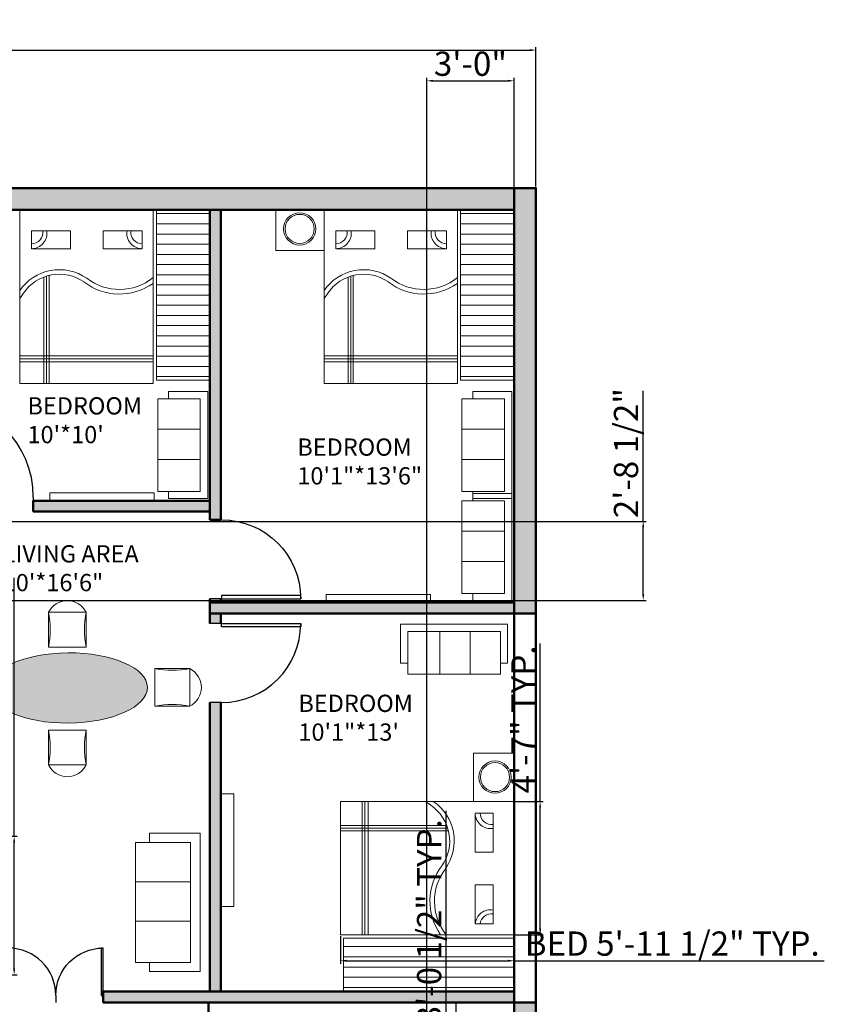
# Model space of a CAD drawing. Units: inches. Extents: x 1477 to 2233, y 1388 to 2326.
# Tile 4 of 4: x 1901 to 2233, y 1870 to 2277. Entities that reach past the tile are written whole.
import ezdxf

# ---------------------------------------------------------------- set-up
doc = ezdxf.new("R2010")
doc.units = ezdxf.units.IN
for name, color, linetype, lineweight in [('A-ANNO-DIMS', 2, 'Continuous', 18), ('A-AREA-IDEN', 7, 'Continuous', 18), ('A-DOOR', 4, 'Continuous', 25), ('A-EQPM', 8, 'Continuous', 18), ('A-FLOR-CASE', 9, 'Continuous', 25), ('A-FURN-PATT', 9, 'Continuous', 13), ('A-WALL-PATT', 10, 'Continuous', 13), ('bed', 200, 'Continuous', 18), ('book', 104, 'Continuous', 18), ('dining', 220, 'Continuous', 18), ('sofa', 130, 'Continuous', 18), ('table', 40, 'Continuous', 18), ('wall', 10, 'Continuous', 50)]:
    doc.layers.add(name, color=color, linetype=linetype, lineweight=lineweight)
doc.styles.get("Standard").update_dxf_attribs({"font": 'arial.ttf'})
doc.dimstyles.new('ISO-25', dxfattribs={"dimtxt": 10, "dimasz": 2.5, "dimexe": 1.25, "dimexo": 0.625, "dimtad": 1, "dimdec": 0, "dimlunit": 4, "dimtxsty": 'Standard', "dimcen": 2.5, "dimadec": 0, "dimazin": 0, "dimtfac": 1, "dimtdec": 0, "dimtmove": 0, "dimatfit": 3, "dimfxl": 1, "dimarcsym": 0})

# ---------------------------------------------------------------- blocks, each defined once
blk = doc.blocks.new('*U2')
for p, q in [((0, 0), (0, -6)), ((40, 0), (40, -6))]:
    blk.add_line(p, q)
blk.add_lwpolyline([(0, 0), (0, 40), (1.75, 40), (1.75, 0)], close=True)
blk.add_arc((0, 0), 40, 0, 90)
blk = doc.blocks.new('*D4')
at = {"layer": 'A-ANNO-DIMS', "color": 0, "lineweight": -2, "transparency": 16777216}
for p, q in [((1601.11, 2207.8), (1601.11, 2265.33)), ((1603.61, 2264.08), (2111.11, 2264.08)), ((2113.61, 2207.8), (2113.61, 2265.33))]:
    blk.add_line(p, q, dxfattribs=at)
at = {"layer": 'A-ANNO-DIMS', "color": 0, "transparency": 16777216}
for points in [[(1603.61, 2264.5), (1603.61, 2263.66), (1601.11, 2264.08)], [(2111.11, 2264.5), (2111.11, 2263.66), (2113.61, 2264.08)]]:
    blk.add_solid(points, dxfattribs=at)
at = {"layer": 'Defpoints', "color": 0, "transparency": 16777216}
for p in [(2113.61, 2264.08), (1601.11, 2207.17), (2113.61, 2207.17)]:
    blk.add_point(p, dxfattribs=at)
at = {"layer": 'A-ANNO-DIMS', "color": 0, "transparency": 16777216, "insert": (1857.36, 2269.81), "char_height": 10, "attachment_point": 5}
blk.add_mtext('42\'-9"', dxfattribs=at)
blk = doc.blocks.new('BED-DOUBLE')
for p, q in [((42.9, 44.24), (42.9, 44.54)), ((42.9, 44.24), (42.9, 0)), ((43.98, 44.24), (43.98, 0)), ((45.09, 43.85), (45.09, 0)), ((53.44, 37.23), (54.99, 35.03)), ((0, 11.42), (54.99, 11.42)), ((0, 10.1), (54.99, 10.1)), ((0, 8.97), (54.99, 8.97))]:
    blk.add_line(p, q)
for points in [[(0, 71.61), (54.99, 71.61), (54.99, 0), (0, 0)], [(4.46, 63.01), (20.6, 63.01), (20.6, 55.57), (4.46, 55.57)], [(50.13, 63.01), (34, 63.01), (34, 55.57), (50.13, 55.57)]]:
    blk.add_lwpolyline(points, close=True)
for centre, radius, start, end in [((4.46, 61.93), 6.36, 270, 9.8305), ((4.46, 62.26), 4.68, 270, 9.2541), ((50.13, 61.93), 6.36, 170.1695, 270), ((50.13, 62.26), 4.68, 170.7459, 270), ((38.65, 27.17), 19.76, 34.2245, 124.798), ((38.65, 27.17), 17.88, 34.2245, 124.798), ((13.85, 60.88), 22.1, 231.1871, 307.7214), ((13.85, 60.88), 23.99, 234.7235, 307.7214)]:
    blk.add_arc(centre, radius, start, end)
blk = doc.blocks.new('BED-DOUBLE-ALT')
for p, q in [((8.97, 0), (8.97, 54.99)), ((10.1, 0), (10.1, 54.99)), ((11.42, 0), (11.42, 54.99)), ((37.23, 53.44), (35.03, 54.99)), ((43.85, 45.09), (0, 45.09)), ((44.24, 43.98), (0, 43.98)), ((44.24, 42.9), (0, 42.9)), ((44.24, 42.9), (44.54, 42.9))]:
    blk.add_line(p, q)
for points in [[(71.61, 0), (71.61, 54.99), (0, 54.99), (0, 0)], [(63.01, 50.13), (63.01, 34), (55.57, 34), (55.57, 50.13)], [(63.01, 4.46), (63.01, 20.6), (55.57, 20.6), (55.57, 4.46)]]:
    blk.add_lwpolyline(points, close=True)
for centre, radius, start, end in [((27.17, 38.65), 17.88, 325.202, 55.7755), ((27.17, 38.65), 19.76, 325.202, 55.7755), ((61.93, 50.13), 6.36, 180, 279.8305), ((62.26, 50.13), 4.68, 180, 279.2541), ((60.88, 13.85), 23.99, 142.2786, 215.2765), ((60.88, 13.85), 22.1, 142.2786, 218.8129), ((61.93, 3.93), 6.36, 80.1695, 175.1865), ((62.26, 3.93), 4.68, 80.7459, 173.4549)]:
    blk.add_arc(centre, radius, start, end)
blk = doc.blocks.new('NIGHTSTAND-LAMP')
blk.add_lwpolyline([(0, 16.8), (19.92, 16.8), (19.92, 0), (0, 0)], close=True)
for radius in [6.66, 6]:
    blk.add_circle((10.02, 8.94), radius)
blk = doc.blocks.new('SOFA-COMPACT-ALT')
for p, q in [((0, 4.5), (0, 20.62)), ((0, 20.62), (44.13, 20.62)), ((44.13, 4.5), (44.13, 20.62)), ((16.11, 17.56), (16.11, 0)), ((28.61, 17.56), (28.61, 0)), ((2.91, 4.5), (0, 4.5)), ((1.29, 4.5), (2.91, 4.5)), ((41.13, 4.5), (44.13, 4.5))]:
    blk.add_line(p, q)
blk.add_lwpolyline([(2.91, 0), (2.91, 17.56), (41.13, 17.56), (41.13, 0)], close=True)
blk = doc.blocks.new('SOFA-STANDARD-ALT')
for p, q in [((0, 26.7), (57.14, 26.7)), ((0, 26.7), (0, 5.83)), ((57.14, 5.83), (57.14, 26.7)), ((20.86, 22.74), (20.86, 0)), ((37.04, 22.74), (37.04, 0)), ((3.76, 5.83), (0, 5.83)), ((53.26, 5.83), (57.14, 5.83))]:
    blk.add_line(p, q)
blk.add_lwpolyline([(3.76, 0), (3.76, 22.74), (53.26, 22.74), (53.26, 0)], close=True)
blk = doc.blocks.new('CHAIR-DINING')
blk.add_lwpolyline([(0, 0), (15.48, 0), (15.48, 14.4), (0, 14.4)], close=True)
for centre, radius, start, end in [((7.74, 10.64), 8.6, 25.8733, 154.1267), ((-38.59, 7.2), 39.26, 349.434, 10.566), ((53.9, 7.2), 39.09, 169.3873, 190.6127)]:
    blk.add_arc(centre, radius, start, end)
blk = doc.blocks.new('*D19')
at = {"layer": 'A-ANNO-DIMS', "color": 0, "lineweight": -2, "transparency": 16777216}
for p, q in [((1898.42, 1939.74), (1898.42, 2046.31)), ((1890.47, 1939.74), (1899.67, 1939.74)), ((1898.42, 1885.1), (1898.42, 1937.24)), ((1890.47, 1882.6), (1899.67, 1882.6))]:
    blk.add_line(p, q, dxfattribs=at)
at = {"layer": 'A-ANNO-DIMS', "color": 0, "transparency": 16777216}
for points in [[(1898, 1937.24), (1898.83, 1937.24), (1898.42, 1939.74)], [(1898, 1885.1), (1898.83, 1885.1), (1898.42, 1882.6)]]:
    blk.add_solid(points, dxfattribs=at)
at = {"layer": 'Defpoints', "color": 0, "transparency": 16777216}
for p in [(1889.85, 1939.74), (1898.42, 1939.74), (1889.85, 1882.6)]:
    blk.add_point(p, dxfattribs=at)
at = {"layer": 'A-ANNO-DIMS', "color": 0, "transparency": 16777216, "insert": (1892.62, 1994.27), "char_height": 10, "attachment_point": 5, "rotation": 90}
blk.add_mtext('SOFA 4\'-9" TYP.', dxfattribs=at)
blk = doc.blocks.new('*D25')
at = {"layer": 'A-ANNO-DIMS', "color": 0, "lineweight": -2, "transparency": 16777216}
for p, q in [((2033, 1898.51), (2033, 1887.14)), ((2104.61, 1898.51), (2104.61, 1887.14)), ((2035.5, 1888.39), (2102.11, 1888.39)), ((2104.61, 1888.39), (2232.55, 1888.39))]:
    blk.add_line(p, q, dxfattribs=at)
at = {"layer": 'A-ANNO-DIMS', "color": 0, "transparency": 16777216}
for points in [[(2035.5, 1888.81), (2035.5, 1887.97), (2033, 1888.39)], [(2102.11, 1888.81), (2102.11, 1887.97), (2104.61, 1888.39)]]:
    blk.add_solid(points, dxfattribs=at)
at = {"layer": 'Defpoints', "color": 0, "transparency": 16777216}
for p in [(2033, 1899.13), (2104.61, 1899.13), (2104.61, 1888.39)]:
    blk.add_point(p, dxfattribs=at)
at = {"layer": 'A-ANNO-DIMS', "color": 0, "transparency": 16777216, "insert": (2169.83, 1894.18), "char_height": 10, "attachment_point": 5}
blk.add_mtext('BED 5\'-11 1/2" TYP.', dxfattribs=at)
blk = doc.blocks.new('*D26')
at = {"layer": 'A-ANNO-DIMS', "color": 0, "lineweight": -2, "transparency": 16777216}
for p, q in [((2115.35, 1954.13), (2115.35, 2019.23)), ((2105.23, 1954.13), (2116.6, 1954.13)), ((2115.35, 1901.63), (2115.35, 1951.63)), ((2105.23, 1899.13), (2116.6, 1899.13))]:
    blk.add_line(p, q, dxfattribs=at)
at = {"layer": 'A-ANNO-DIMS', "color": 0, "transparency": 16777216}
for points in [[(2114.93, 1951.63), (2115.77, 1951.63), (2115.35, 1954.13)], [(2114.93, 1901.63), (2115.77, 1901.63), (2115.35, 1899.13)]]:
    blk.add_solid(points, dxfattribs=at)
at = {"layer": 'Defpoints', "color": 0, "transparency": 16777216}
for p in [(2104.61, 1954.13), (2115.35, 1954.13), (2104.61, 1899.13)]:
    blk.add_point(p, dxfattribs=at)
at = {"layer": 'A-ANNO-DIMS', "color": 0, "transparency": 16777216, "insert": (2109.72, 1987.93), "char_height": 10, "attachment_point": 5, "rotation": 90}
blk.add_mtext('4\'-7" TYP.', dxfattribs=at)
blk = doc.blocks.new('*D29')
at = {"layer": 'A-ANNO-DIMS', "color": 0, "lineweight": -2, "transparency": 16777216}
for p, q in [((2076.64, 1799.12), (2076.64, 1950.21)), ((2081.48, 1799.12), (2075.39, 1799.12)), ((2076.64, 1765.24), (2076.64, 1796.62)), ((2081.48, 1762.74), (2075.39, 1762.74))]:
    blk.add_line(p, q, dxfattribs=at)
at = {"layer": 'A-ANNO-DIMS', "color": 0, "transparency": 16777216}
for points in [[(2076.23, 1796.62), (2077.06, 1796.62), (2076.64, 1799.12)], [(2076.23, 1765.24), (2077.06, 1765.24), (2076.64, 1762.74)]]:
    blk.add_solid(points, dxfattribs=at)
at = {"layer": 'Defpoints', "color": 0, "transparency": 16777216}
for p in [(2076.64, 1799.12), (2082.1, 1799.12), (2082.1, 1762.74)]:
    blk.add_point(p, dxfattribs=at)
at = {"layer": 'A-ANNO-DIMS', "color": 0, "transparency": 16777216, "insert": (2070.85, 1875.92), "char_height": 10, "attachment_point": 5, "rotation": 90}
blk.add_mtext('FIXTURE 3\'-0 1/2" TYP.', dxfattribs=at)
blk = doc.blocks.new('*D35')
at = {"layer": 'A-ANNO-DIMS', "color": 0, "lineweight": -2, "transparency": 16777216}
for p, q in [((2068.61, 1625.95), (2068.61, 2252.67)), ((2071.11, 2251.42), (2102.11, 2251.42)), ((2104.61, 1625.66), (2104.61, 2252.67))]:
    blk.add_line(p, q, dxfattribs=at)
at = {"layer": 'A-ANNO-DIMS', "color": 0, "transparency": 16777216}
for points in [[(2071.11, 2251.84), (2071.11, 2251.01), (2068.61, 2251.42)], [(2102.11, 2251.84), (2102.11, 2251.01), (2104.61, 2251.42)]]:
    blk.add_solid(points, dxfattribs=at)
at = {"layer": 'Defpoints', "color": 0, "transparency": 16777216}
for p in [(2104.61, 2251.42), (2068.61, 1625.33), (2104.61, 1625.03)]:
    blk.add_point(p, dxfattribs=at)
at = {"layer": 'A-ANNO-DIMS', "color": 0, "transparency": 16777216, "insert": (2086.61, 2257.16), "char_height": 10, "attachment_point": 5}
blk.add_mtext('3\'-0"', dxfattribs=at)
blk = doc.blocks.new('*D37')
at = {"layer": 'A-ANNO-DIMS', "color": 0, "lineweight": -2, "transparency": 16777216}
for p, q in [((2080.61, 1870.55), (2080.61, 1395.67)), ((2104.61, 1870.55), (2104.61, 1395.67)), ((2083.11, 1396.92), (2102.11, 1396.92)), ((2104.61, 1396.92), (2135.11, 1396.92))]:
    blk.add_line(p, q, dxfattribs=at)
at = {"layer": 'A-ANNO-DIMS', "color": 0, "transparency": 16777216}
for points in [[(2083.11, 1397.34), (2083.11, 1396.51), (2080.61, 1396.92)], [(2102.11, 1397.34), (2102.11, 1396.51), (2104.61, 1396.92)]]:
    blk.add_solid(points, dxfattribs=at)
at = {"layer": 'Defpoints', "color": 0, "transparency": 16777216}
for p in [(2080.61, 1871.17), (2104.61, 1871.17), (2104.61, 1396.92)]:
    blk.add_point(p, dxfattribs=at)
at = {"layer": 'A-ANNO-DIMS', "color": 0, "transparency": 16777216, "insert": (2121.11, 1402.65), "char_height": 10, "attachment_point": 5}
blk.add_mtext('2\'-0"', dxfattribs=at)
blk = doc.blocks.new('*D40')
at = {"layer": 'A-ANNO-DIMS', "color": 0, "lineweight": -2, "transparency": 16777216}
for p, q in [((2157.86, 2069.66), (2157.86, 2123.47)), ((1730.73, 2069.66), (2159.11, 2069.66)), ((2157.86, 2039.56), (2157.86, 2067.16)), ((1730.73, 2037.06), (2159.11, 2037.06))]:
    blk.add_line(p, q, dxfattribs=at)
at = {"layer": 'A-ANNO-DIMS', "color": 0, "transparency": 16777216}
for points in [[(2157.44, 2067.16), (2158.27, 2067.16), (2157.86, 2069.66)], [(2157.44, 2039.56), (2158.27, 2039.56), (2157.86, 2037.06)]]:
    blk.add_solid(points, dxfattribs=at)
at = {"layer": 'Defpoints', "color": 0, "transparency": 16777216}
for p in [(1730.11, 2069.66), (2157.86, 2069.66), (1730.11, 2037.06)]:
    blk.add_point(p, dxfattribs=at)
at = {"layer": 'A-ANNO-DIMS', "color": 0, "transparency": 16777216, "insert": (2152.06, 2097.82), "char_height": 10, "attachment_point": 5, "rotation": 90}
blk.add_mtext('2\'-8 1/2"', dxfattribs=at)

msp = doc.modelspace()

# ---------------------------------------------------------------- hatches: boundary and pattern name
at = {"layer": 'A-FURN-PATT'}
h = msp.add_hatch(dxfattribs=at)
h.set_pattern_fill('_USER', color=256, scale=4.2, pattern_type=0)
h.set_pattern_definition([(0, (0, 0), (0, 4.2), [])])
h.paths.add_polyline_path([(1632.2, 2197.32), (1610.11, 2197.32), (1610.11, 2127.01), (1632.2, 2127.01)])
h.paths.add_polyline_path([(1757.03, 2198.17), (1734.93, 2198.17), (1734.93, 2127.87), (1757.03, 2127.87)])
h.paths.add_polyline_path([(1979.11, 2198.17), (1957.06, 2198.17), (1957.06, 2127.87), (1979.11, 2127.87)])
h.paths.add_polyline_path([(2104.61, 2198.17), (2082.56, 2198.17), (2082.56, 2127.87), (2104.61, 2127.87)])
h.paths.add_polyline_path([(2104.61, 1897.77), (2034.3, 1897.77), (2034.3, 1875.67), (2104.61, 1875.67)])
h.paths.add_polyline_path([(1680.41, 1898.15), (1610.11, 1898.15), (1610.11, 1876.06), (1680.41, 1876.06)])
h.paths.add_polyline_path([(1680.41, 1869.67), (1610.11, 1869.67), (1610.11, 1847.57), (1680.41, 1847.57)])
h.paths.add_polyline_path([(1632.2, 1521.19), (1610.11, 1521.19), (1610.11, 1450.88), (1632.2, 1450.88)])
h.paths.add_polyline_path([(1854.34, 1520.43), (1832.24, 1520.43), (1832.24, 1450.17), (1854.34, 1450.17)])
h = msp.add_hatch(color=256, dxfattribs=at)
h.dxf.hatch_style = 1
edge = h.paths.add_edge_path()
edge.add_ellipse((1794.61, 1999.29), major_axis=(32.65, 0.27), ratio=0.443592, start_angle=0, end_angle=360)
edge = h.paths.add_edge_path()
edge.add_ellipse((1920.72, 2000.93), major_axis=(32.65, 0.27), ratio=0.443592, start_angle=0, end_angle=360)
edge = h.paths.add_edge_path()
edge.add_ellipse((1854.61, 1811.96), major_axis=(32.65, 0.27), ratio=0.443592, start_angle=0, end_angle=360)
edge = h.paths.add_edge_path()
edge.add_ellipse((1749.3, 1659.55), major_axis=(32.65, 0.27), ratio=0.443592, start_angle=0, end_angle=360)
at = {"layer": 'A-WALL-PATT'}
h = msp.add_hatch(color=256, dxfattribs=at)
h.dxf.hatch_style = 1
h.paths.add_polyline_path([(2104.61, 2036.17), (1979.11, 2036.17), (1979.11, 2031.67), (2104.61, 2031.67)])
h.paths.add_polyline_path([(1983.61, 2031.67), (1979.11, 2031.67), (1979.11, 2027.53), (1983.61, 2027.53)])
h.paths.add_polyline_path([(1983.61, 2037.7), (1979.11, 2037.7), (1979.11, 2036.17), (1983.61, 2036.17)])
h.paths.add_polyline_path([(2113.61, 2207.17), (2104.61, 2207.17), (2104.61, 2031.67), (2113.61, 2031.67)])
h.paths.add_polyline_path([(2104.61, 2207.17), (1859.11, 2207.17), (1859.11, 2198.17), (2104.61, 2198.17)])
h.paths.add_polyline_path([(1983.61, 2198.17), (1979.16, 2198.17), (1979.16, 2127.87), (1979.11, 2070.31), (1983.61, 2070.31)])
h.paths.add_polyline_path([(1979.11, 2078.17), (1906.33, 2078.17), (1906.33, 2073.67), (1979.11, 2073.67)])
h.paths.add_polyline_path([(1859.11, 2198.17), (1854.61, 2198.17), (1854.61, 2078.17), (1859.11, 2078.17)])
h.paths.add_polyline_path([(1866.33, 2078.17), (1848.79, 2078.17), (1848.79, 2073.67), (1866.33, 2073.67)])
h.paths.add_polyline_path([(1859.11, 2207.17), (1734.61, 2207.17), (1734.61, 2198.17), (1859.11, 2198.17)])
h.paths.add_polyline_path([(1734.61, 2207.17), (1601.11, 2207.17), (1601.11, 2198.17), (1610.11, 2198.17), (1734.61, 2198.17)])
h.paths.add_polyline_path([(1734.61, 2198.17), (1730.11, 2198.17), (1730.11, 2069.66), (1734.61, 2069.66)])
h.paths.add_polyline_path([(1808.79, 2078.17), (1734.61, 2078.17), (1734.61, 2073.67), (1808.79, 2073.67)])
h.paths.add_polyline_path([(1610.11, 2198.17), (1601.11, 2198.17), (1601.11, 1450.43), (1610.11, 1450.43)])
h.paths.add_polyline_path([(2104.61, 1450.43), (1854.61, 1450.43), (1854.61, 1450.17), (1854.34, 1450.13), (1832.24, 1450.13), (1830.34, 1450.13), (1830.34, 1450.03), (1775.35, 1450.03), (1755.43, 1450.03), (1713.79, 1450.14), (1713.79, 1450.03), (1693.87, 1450.03), (1638.87, 1450.03), (1610.11, 1450.17), (1610.11, 1450.43), (1601.11, 1450.43), (1601.11, 1441.17), (2104.61, 1441.17)])
h.paths.add_polyline_path([(2113.61, 1871.17), (2104.61, 1871.17), (2104.61, 1441.17), (2113.61, 1441.17)])
h.paths.add_polyline_path([(1734.61, 1598.17), (1730.11, 1598.17), (1730.11, 1450.43), (1734.61, 1450.43)])
h = msp.add_hatch(color=256, dxfattribs=at)
h.dxf.hatch_style = 1
h.paths.add_polyline_path([(1734.61, 2037.06), (1730.11, 2037.06), (1730.11, 2036.17), (1610.11, 2036.17), (1610.11, 2031.67), (1734.61, 2031.67)])
h.paths.add_polyline_path([(1983.61, 1994.92), (1979.11, 1994.92), (1979.11, 1875.67), (1983.61, 1875.67)])
h = msp.add_hatch(color=256, dxfattribs=at)
h.dxf.hatch_style = 1
h.paths.add_polyline_path([(1734.61, 1993.71), (1730.11, 1993.71), (1730.11, 1875.67), (1734.61, 1875.67)])
h.paths.add_polyline_path([(1730.11, 1875.67), (1610.11, 1875.67), (1610.11, 1871.17), (1730.11, 1871.17)])
h.paths.add_polyline_path([(1776.57, 1875.67), (1730.11, 1875.67), (1730.11, 1871.17), (1776.57, 1871.17)])
h.paths.add_polyline_path([(1896.07, 1875.67), (1815.6, 1875.67), (1815.6, 1871.17), (1896.07, 1871.17)])
h.paths.add_polyline_path([(2104.61, 1875.67), (1935.11, 1875.67), (1935.11, 1871.17), (2104.61, 1871.17)])
h.paths.add_polyline_path([(1734.61, 1871.17), (1730.11, 1871.17), (1730.11, 1727.17), (1734.61, 1727.17)])
h.paths.add_polyline_path([(1775, 1727.17), (1726.93, 1727.17), (1726.93, 1722.67), (1775, 1722.67)])
h.paths.add_polyline_path([(1880.17, 1727.17), (1814.04, 1727.17), (1814.04, 1722.67), (1880.17, 1722.67)])
h.paths.add_polyline_path([(1858.61, 1722.67), (1854.11, 1722.67), (1854.12, 1598.17), (1858.61, 1598.17)])
h.paths.add_polyline_path([(1854.12, 1602.67), (1780.08, 1602.67), (1780.08, 1598.17), (1854.12, 1598.17)])
h.paths.add_polyline_path([(1740.08, 1602.67), (1722.89, 1602.67), (1722.89, 1598.17), (1740.08, 1598.17)])
h.paths.add_polyline_path([(1682.89, 1602.67), (1610.11, 1602.67), (1610.11, 1598.17), (1682.89, 1598.17)])
h.paths.add_polyline_path([(1859.11, 1598.17), (1854.61, 1598.17), (1854.61, 1450.43), (1859.11, 1450.43)])
h.paths.add_polyline_path([(2104.61, 1727.17), (1960.17, 1727.17), (1960.17, 1722.67), (2104.61, 1722.67)])
h.paths.add_polyline_path([(2104.61, 1625.03), (1978.61, 1625.03), (1978.61, 1620.53), (2104.61, 1620.53)])

# ---------------------------------------------------------------- linework, layer by layer
at = {"layer": 'A-EQPM'}
for points in [[(1956.17, 2078.17), (1913.12, 2078.17), (1913.12, 2081.42), (1956.17, 2081.42)], [(2070.17, 2036.17), (2027.12, 2036.17), (2027.12, 2039.42), (2070.17, 2039.42)], [(1983.91, 1910.78), (1989.01, 1910.78), (1989.01, 1957.26), (1983.91, 1957.26)]]:
    msp.add_lwpolyline(points, close=True, dxfattribs=at)
at = {"layer": 'A-FLOR-CASE'}
for p, q in [((2104.61, 1871.17), (2080.61, 1871.17)), ((2080.61, 1871.17), (2080.61, 1751.17))]:
    msp.add_line(p, q, dxfattribs=at)
at = {"layer": 'book'}
for points in [[(1957.06, 2198.17), (1979.16, 2198.17), (1979.16, 2127.87), (1957.06, 2127.87)], [(2082.56, 2198.17), (2104.66, 2198.17), (2104.66, 2127.87), (2082.56, 2127.87)], [(2104.61, 1897.77), (2104.61, 1875.67), (2034.3, 1875.67), (2034.3, 1897.77)]]:
    msp.add_lwpolyline(points, close=True, dxfattribs=at)
at = {"layer": 'dining'}
msp.add_ellipse((1920.72, 2000.93), major_axis=(32.65, 0.27), ratio=0.443592, dxfattribs=at)
at = {"layer": 'wall'}
for p, q in [((1859.11, 2207.17), (1983.61, 2207.17)), ((1983.61, 2207.17), (2113.61, 2207.17)), ((2113.61, 2207.17), (2113.61, 2031.67)), ((1859.11, 2198.17), (1979.11, 2198.17)), ((1979.11, 2198.17), (1979.11, 2078.17)), ((1983.61, 2198.17), (1983.61, 2073.67)), ((1983.61, 2198.17), (2104.61, 2198.17)), ((2104.61, 2198.17), (2104.61, 2036.17)), ((1979.11, 2078.17), (1979.11, 2120.13)), ((1983.61, 2070.31), (1983.61, 2120.13)), ((1979.11, 2078.17), (1906.33, 2078.17)), ((1979.11, 2073.67), (1906.33, 2073.67)), ((1979.11, 2070.31), (1979.11, 2073.67)), ((1979.11, 2031.67), (1979.11, 2037.7)), ((1983.61, 2036.17), (1983.61, 2037.7)), ((2104.61, 2036.17), (1983.61, 2036.17)), ((2113.61, 2031.67), (1979.11, 2031.67)), ((1979.11, 2027.53), (1979.11, 2031.67)), ((1983.61, 2027.53), (1983.61, 2031.67)), ((2104.61, 2031.67), (2104.61, 1875.67)), ((2113.61, 2031.67), (2113.61, 1871.17)), ((1979.11, 1875.67), (1979.11, 1994.92)), ((1983.61, 1875.67), (1983.61, 1994.92)), ((1915.53, 1875.67), (1915.65, 1875.67)), ((1934.25, 1875.67), (1993.21, 1875.67)), ((2104.61, 1875.67), (1983.61, 1875.67)), ((1935.11, 1871.17), (1981.94, 1871.17)), ((1978.61, 1727.17), (1978.61, 1871.17)), ((2113.61, 1871.17), (1979.11, 1871.17)), ((2104.61, 1871.17), (2104.61, 1727.17)), ((2113.61, 1871.17), (2113.61, 1722.67))]:
    msp.add_line(p, q, dxfattribs=at)
for points in [[(1601.11, 2207.17), (2104.61, 2207.17), (2104.61, 2198.17), (1601.11, 2198.17)], [(2104.61, 2207.17), (2113.61, 2207.17), (2113.61, 1441.17), (2104.61, 1441.17)], [(1979.11, 2070.31), (1983.61, 2070.31), (1983.61, 2198.17), (1979.11, 2198.17)], [(1906.33, 2073.67), (1979.11, 2073.67), (1979.11, 2078.17), (1906.33, 2078.17)], [(1979.11, 2031.67), (2104.61, 2031.67), (2104.61, 2036.17), (1979.11, 2036.17)], [(1935.11, 1871.17), (2104.61, 1871.17), (2104.61, 1875.67), (1935.11, 1875.67)]]:
    msp.add_lwpolyline(points, close=True, dxfattribs=at)

# ---------------------------------------------------------------- block references
at = {"layer": 'A-DOOR'}
msp.add_blockref('*U2', (1866.33, 2079.67), dxfattribs=at)
at = {"layer": 'A-DOOR', "yscale": 0.8152383750006338, "zscale": 0.8152383750006338, "rotation": 270}
for p, xscale in [((1984, 2037.7), -0.8152383750006338), ((1984, 2027.53), 0.8152383750006338)]:
    msp.add_blockref('*U2', p, dxfattribs=dict(at, xscale=xscale))
at = {"layer": 'A-DOOR', "yscale": 0.4878891377503276, "zscale": 0.4878891377503276}
for p, xscale in [((1896.07, 1874.1), 0.4878891377503276), ((1935.11, 1874.1), -0.4878891377503276)]:
    msp.add_blockref('*U2', p, dxfattribs=dict(at, xscale=xscale))
at = {"layer": 'bed', "extrusion": (0, 0, -1), "zscale": -1}
for p in [(-1955.7, 2126.56), (-2081.2, 2126.56)]:
    msp.add_blockref('BED-DOUBLE', p, dxfattribs=at)
at = {"layer": 'bed'}
msp.add_blockref('BED-DOUBLE-ALT', (2033, 1899.13), dxfattribs=at)
at = {"layer": 'dining'}
msp.add_blockref('CHAIR-DINING', (1912.62, 2017.75), dxfattribs=at)
at = {"layer": 'dining', "rotation": 270.0000000000008}
msp.add_blockref('CHAIR-DINING', (1956.43, 2008.9), dxfattribs=at)
at = {"layer": 'dining', "extrusion": (0, 0, -1), "zscale": -1, "rotation": 180}
msp.add_blockref('CHAIR-DINING', (-1912.62, 1983.55), dxfattribs=at)
at = {"layer": 'sofa', "extrusion": (0, 0, -1), "zscale": -1}
for name, p, rotation in [('SOFA-COMPACT-ALT', (-1957.61, 2079.1), 90.00000000000003), ('SOFA-COMPACT-ALT', (-2083.11, 2079.1), 89.99999999999913), ('SOFA-COMPACT-ALT', (-2083.11, 2036.98), 89.99999999999913), ('SOFA-STANDARD-ALT', (-1948.43, 1883.92), 90.00000000000003)]:
    msp.add_blockref(name, p, dxfattribs=dict(at, rotation=rotation))
at = {"layer": 'sofa'}
msp.add_blockref('SOFA-COMPACT-ALT', (2057.82, 2006.6), dxfattribs=at)
at = {"layer": 'table', "extrusion": (0, 0, -1), "zscale": -1}
msp.add_blockref('NIGHTSTAND-LAMP', (-2026.21, 2181.38), dxfattribs=at)
at = {"layer": 'table', "extrusion": (0, 0, -1), "zscale": -1, "rotation": 89.99999999999925}
msp.add_blockref('NIGHTSTAND-LAMP', (-2087.81, 1954.13), dxfattribs=at)

# ---------------------------------------------------------------- texts
at = {"layer": 'A-AREA-IDEN', "attachment_point": 1}
for s, insert, char_height in [("BEDROOM\\P10'*10'", (1903.91, 2120.87), 7.116), ('BEDROOM\\P10\'1"*13\'6"', (2015.2, 2103.86), 7.1161), ('LIVING AREA\\P10\'*16\'6"', (1893.69, 2059.82), 7.1161), ('BEDROOM\\P10\'1"*13\'', (2015.64, 1998.15), 7.116)]:
    msp.add_mtext_dynamic_manual_height_columns(s, width=109.5726, gutter_width=35.58, heights=[0], dxfattribs=dict(at, insert=insert, char_height=char_height))

# ---------------------------------------------------------------- dimensions: what is measured, and where the dimension line sits
at = {"layer": 'A-ANNO-DIMS'}
for base, p1, p2, override, picture, middle in [((2113.60751576, 2264.08102566), (1601.10751576, 2207.17284154), (2113.60751576, 2207.17284154), {"dimclrd": 0, "dimclre": 0, "dimclrt": 0}, '*D4', (1857.35751576, 2269.81175554)), ((2104.61, 2251.42), (2068.61, 1625.33), (2104.61, 1625.03), {"dimdec": 1, "dimlfac": 1, "dimrnd": 0, "dimzin": 1, "dimdsep": 46, "dimlunit": 4, "dimfrac": 2}, '*D35', (2086.61, 2257.16)), ((2104.61, 1396.92), (2080.61, 1871.17), (2104.61, 1871.17), {"dimdec": 1, "dimlfac": 1, "dimrnd": 0, "dimzin": 1, "dimdsep": 46, "dimlunit": 4, "dimfrac": 2}, '*D37', (2121.11, 1402.65))]:
    dim = msp.add_linear_dim(base=base, p1=p1, p2=p2, dimstyle='ISO-25', override=override, dxfattribs=at)
    dim.commit()
    dim.dimension.update_dxf_attribs({"geometry": picture, "text_midpoint": middle})
dim = msp.add_linear_dim(base=(2157.86, 2069.66), p1=(1730.11, 2037.06), p2=(1730.11, 2069.66), angle=90, dimstyle='ISO-25', override={"dimdec": 1, "dimlfac": 1, "dimrnd": 0, "dimzin": 1, "dimdsep": 46, "dimlunit": 4, "dimfrac": 2}, dxfattribs=at)
dim.commit()
dim.dimension.update_dxf_attribs({"geometry": '*D40', "text_midpoint": (2152.06, 2097.82)})
for base, p1, p2, text, picture, middle in [((1898.42, 1939.74), (1889.85, 1882.6), (1889.85, 1939.74), 'SOFA <> TYP.', '*D19', (1892.62, 1994.27)), ((2115.35, 1954.13), (2104.61, 1899.13), (2104.61, 1954.13), '<> TYP.', '*D26', (2109.72, 1987.93)), ((2076.64, 1799.12), (2082.1, 1762.74), (2082.1, 1799.12), 'FIXTURE <> TYP.', '*D29', (2070.85, 1875.92))]:
    dim = msp.add_linear_dim(base=base, p1=p1, p2=p2, angle=90, text=text, dimstyle='ISO-25', override={"dimdec": 1, "dimlfac": 1, "dimrnd": 0, "dimzin": 1, "dimdsep": 46, "dimlunit": 4, "dimfrac": 2}, dxfattribs=at)
    dim.commit()
    dim.dimension.update_dxf_attribs({"geometry": picture, "text_midpoint": middle})
dim = msp.add_linear_dim(base=(2104.61, 1888.39), p1=(2033, 1899.13), p2=(2104.61, 1899.13), text='BED <> TYP.', dimstyle='ISO-25', override={"dimdec": 1, "dimlfac": 1, "dimrnd": 0, "dimzin": 1, "dimdsep": 46, "dimlunit": 4, "dimfrac": 2}, dxfattribs=at)
dim.commit()
dim.dimension.update_dxf_attribs({"geometry": '*D25', "text_midpoint": (2169.83, 1894.18)})

doc.saveas('drawing.dxf')
